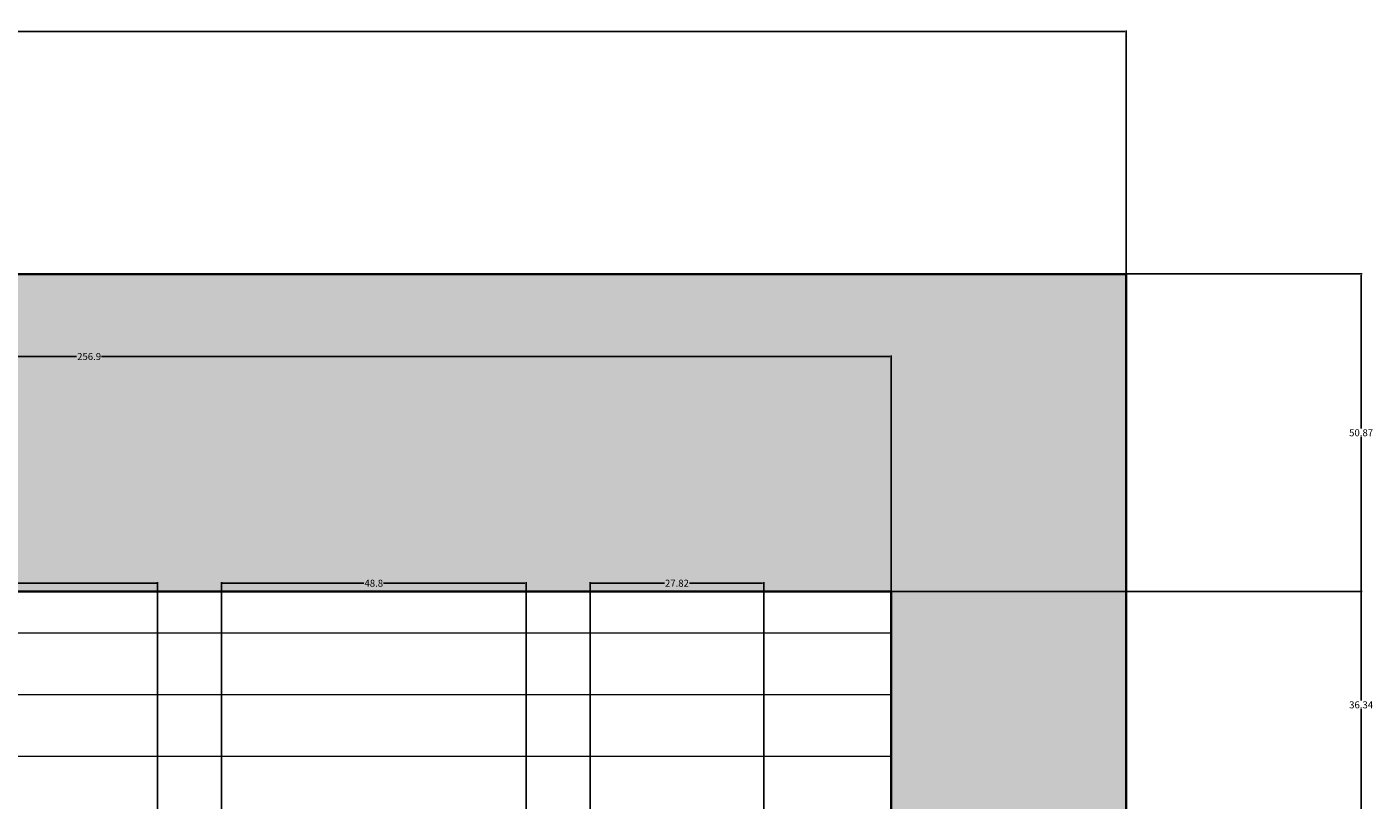
# Model space of a CAD drawing. Units: inches. Extents: x 8 to 634, y 41 to 867.
# Tile 21 of 21: x 418 to 634, y 743 to 867. Entities that reach past the tile are written whole.
import ezdxf

# ---------------------------------------------------------------- set-up
doc = ezdxf.new("R2010")
doc.units = ezdxf.units.IN
doc.header["$MEASUREMENT"] = 0
for name, color, linetype, lineweight in [('A-ANNO-DIMS', 2, 'Continuous', 18), ('A-ROOF', 7, 'Continuous', 35), ('A-ROOF-PATT', 8, 'Continuous', 9), ('A-WALL-PATT', 8, 'Continuous', 9)]:
    doc.layers.add(name, color=color, linetype=linetype, lineweight=lineweight)
doc.styles.get("Standard").update_dxf_attribs({"font": 'arial.ttf'})
doc.dimstyles.get("Standard").update_dxf_attribs({"dimtxt": 1.125, "dimasz": 0.18, "dimexe": 0.18, "dimexo": 0.0625, "dimgap": 0.09, "dimtad": 0, "dimtih": 1, "dimtoh": 1, "dimdec": 4, "dimzin": 0, "dimdsep": 46, "dimlunit": 4, "dimtxsty": 'Standard', "dimcen": 0.09, "dimadec": 0, "dimazin": 0, "dimtfac": 1, "dimtdec": 4, "dimtofl": 0, "dimtmove": 0, "dimatfit": 3, "dimfxl": 1, "dimtolj": 1, "dimtzin": 0, "dimarcsym": 0})

# ---------------------------------------------------------------- blocks, each defined once
blk = doc.blocks.new('*D19')
at = {"layer": 'A-ANNO-DIMS', "color": 0, "lineweight": -2, "transparency": 16777216}
for p, q in [((47.34, 697.73), (47.34, 866.81)), ((47.52, 866.63), (319.51, 866.63)), ((594.17, 866.63), (322.18, 866.63)), ((594.35, 827.83), (594.35, 866.81))]:
    blk.add_line(p, q, dxfattribs=at)
at = {"layer": 'A-ANNO-DIMS', "color": 0, "transparency": 16777216}
for points in [[(47.52, 866.66), (47.52, 866.6), (47.34, 866.63)], [(594.17, 866.66), (594.17, 866.6), (594.35, 866.63)]]:
    blk.add_solid(points, dxfattribs=at)
at = {"layer": 'Defpoints', "color": 0, "transparency": 16777216}
for p in [(594.35, 866.63), (594.35, 827.77), (47.34, 697.67)]:
    blk.add_point(p, dxfattribs=at)
at = {"layer": 'A-ANNO-DIMS', "color": 0, "transparency": 16777216, "insert": (320.85, 866.63), "char_height": 1.125, "attachment_point": 5}
blk.add_mtext('\\A1;547', dxfattribs=at)
blk = doc.blocks.new('*D45')
at = {"layer": 'A-ANNO-DIMS', "color": 0, "lineweight": -2, "transparency": 16777216}
for p, q in [((556.77, 776.89), (632.18, 776.89)), ((632, 776.71), (632, 759.39)), ((632, 740.74), (632, 758.06)), ((536.38, 740.56), (632.18, 740.56))]:
    blk.add_line(p, q, dxfattribs=at)
at = {"layer": 'A-ANNO-DIMS', "color": 0, "transparency": 16777216}
for points in [[(631.97, 776.71), (632.03, 776.71), (632, 776.89)], [(631.97, 740.74), (632.03, 740.74), (632, 740.56)]]:
    blk.add_solid(points, dxfattribs=at)
at = {"layer": 'Defpoints', "color": 0, "transparency": 16777216}
for p in [(556.71, 776.89), (632, 776.89), (536.32, 740.56)]:
    blk.add_point(p, dxfattribs=at)
at = {"layer": 'A-ANNO-DIMS', "color": 0, "transparency": 16777216, "insert": (632, 758.72), "char_height": 1.125, "attachment_point": 5}
blk.add_mtext('\\A1;36.34', dxfattribs=at)
blk = doc.blocks.new('*D46')
at = {"layer": 'A-ANNO-DIMS', "color": 0, "lineweight": -2, "transparency": 16777216}
for p, q in [((594.41, 827.77), (632.18, 827.77)), ((632, 827.59), (632, 802.99)), ((632, 777.07), (632, 801.67)), ((556.77, 776.89), (632.18, 776.89))]:
    blk.add_line(p, q, dxfattribs=at)
at = {"layer": 'A-ANNO-DIMS', "color": 0, "transparency": 16777216}
for points in [[(631.97, 827.59), (632.03, 827.59), (632, 827.77)], [(631.97, 777.07), (632.03, 777.07), (632, 776.89)]]:
    blk.add_solid(points, dxfattribs=at)
at = {"layer": 'Defpoints', "color": 0, "transparency": 16777216}
for p in [(594.35, 827.77), (632, 827.77), (556.71, 776.89)]:
    blk.add_point(p, dxfattribs=at)
at = {"layer": 'A-ANNO-DIMS', "color": 0, "transparency": 16777216, "insert": (632, 802.33), "char_height": 1.125, "attachment_point": 5}
blk.add_mtext('\\A1;50.87', dxfattribs=at)
blk = doc.blocks.new('*D47')
at = {"layer": 'A-ANNO-DIMS', "color": 0, "lineweight": -2, "transparency": 16777216}
for p, q in [((299.8, 776.96), (299.8, 814.72)), ((299.98, 814.54), (426.25, 814.54)), ((556.53, 814.54), (430.25, 814.54)), ((556.71, 776.96), (556.71, 814.72))]:
    blk.add_line(p, q, dxfattribs=at)
at = {"layer": 'A-ANNO-DIMS', "color": 0, "transparency": 16777216}
for points in [[(299.98, 814.57), (299.98, 814.51), (299.8, 814.54)], [(556.53, 814.57), (556.53, 814.51), (556.71, 814.54)]]:
    blk.add_solid(points, dxfattribs=at)
at = {"layer": 'Defpoints', "color": 0, "transparency": 16777216}
for p in [(556.71, 814.54), (299.8, 776.89), (556.71, 776.89)]:
    blk.add_point(p, dxfattribs=at)
at = {"layer": 'A-ANNO-DIMS', "color": 0, "transparency": 16777216, "insert": (428.25, 814.54), "char_height": 1.125, "attachment_point": 5}
blk.add_mtext('\\A1;256.9', dxfattribs=at)
blk = doc.blocks.new('*D50')
at = {"layer": 'A-ANNO-DIMS', "color": 0, "lineweight": -2, "transparency": 16777216}
for p, q in [((370.39, 740.62), (370.39, 778.39)), ((370.57, 778.21), (402.91, 778.21)), ((439.02, 778.21), (406.68, 778.21)), ((439.2, 740.62), (439.2, 778.39))]:
    blk.add_line(p, q, dxfattribs=at)
at = {"layer": 'A-ANNO-DIMS', "color": 0, "transparency": 16777216}
for points in [[(370.57, 778.24), (370.57, 778.18), (370.39, 778.21)], [(439.02, 778.24), (439.02, 778.18), (439.2, 778.21)]]:
    blk.add_solid(points, dxfattribs=at)
at = {"layer": 'Defpoints', "color": 0, "transparency": 16777216}
for p in [(439.2, 778.21), (370.39, 740.56), (439.2, 740.56)]:
    blk.add_point(p, dxfattribs=at)
at = {"layer": 'A-ANNO-DIMS', "color": 0, "transparency": 16777216, "insert": (404.79, 778.21), "char_height": 1.125, "attachment_point": 5}
blk.add_mtext('\\A1;68.81', dxfattribs=at)
blk = doc.blocks.new('*D52')
at = {"layer": 'A-ANNO-DIMS', "color": 0, "lineweight": -2, "transparency": 16777216}
for p, q in [((449.45, 740.62), (449.45, 778.39)), ((449.63, 778.21), (472.28, 778.21)), ((498.07, 778.21), (475.43, 778.21)), ((498.25, 740.62), (498.25, 778.39))]:
    blk.add_line(p, q, dxfattribs=at)
at = {"layer": 'A-ANNO-DIMS', "color": 0, "transparency": 16777216}
for points in [[(449.63, 778.24), (449.63, 778.18), (449.45, 778.21)], [(498.07, 778.24), (498.07, 778.18), (498.25, 778.21)]]:
    blk.add_solid(points, dxfattribs=at)
at = {"layer": 'Defpoints', "color": 0, "transparency": 16777216}
for p in [(498.25, 778.21), (449.45, 740.56), (498.25, 740.56)]:
    blk.add_point(p, dxfattribs=at)
at = {"layer": 'A-ANNO-DIMS', "color": 0, "transparency": 16777216, "insert": (473.85, 778.21), "char_height": 1.125, "attachment_point": 5}
blk.add_mtext('\\A1;48.8', dxfattribs=at)
blk = doc.blocks.new('*D54')
at = {"layer": 'A-ANNO-DIMS', "color": 0, "lineweight": -2, "transparency": 16777216}
for p, q in [((508.5, 740.62), (508.5, 778.39)), ((508.68, 778.21), (520.42, 778.21)), ((536.14, 778.21), (524.4, 778.21)), ((536.32, 740.62), (536.32, 778.39))]:
    blk.add_line(p, q, dxfattribs=at)
at = {"layer": 'A-ANNO-DIMS', "color": 0, "transparency": 16777216}
for points in [[(508.68, 778.24), (508.68, 778.18), (508.5, 778.21)], [(536.14, 778.24), (536.14, 778.18), (536.32, 778.21)]]:
    blk.add_solid(points, dxfattribs=at)
at = {"layer": 'Defpoints', "color": 0, "transparency": 16777216}
for p in [(536.32, 778.21), (508.5, 740.56), (536.32, 740.56)]:
    blk.add_point(p, dxfattribs=at)
at = {"layer": 'A-ANNO-DIMS', "color": 0, "transparency": 16777216, "insert": (522.41, 778.21), "char_height": 1.125, "attachment_point": 5}
blk.add_mtext('\\A1;27.82', dxfattribs=at)

msp = doc.modelspace()

# ---------------------------------------------------------------- hatches: boundary and pattern name
at = {"layer": 'A-ROOF-PATT', "transparency": 33554687}
h = msp.add_hatch(dxfattribs=at)
h.set_pattern_fill('AR-CONC', color=256, scale=2.2, angle=135)
h.paths.add_polyline_path([(262.2266, 828.9821), (144.3564, 828.9821), (144.3564, 697.6655), (262.2266, 785.231), (245.114, 785.231), (245.114, 792.8938), (262.2266, 792.8938)])
h.paths.add_polyline_path([(594.3501, 827.7671), (262.2266, 827.7671), (262.2266, 792.8938), (262.2266, 697.6655), (299.7961, 697.6655), (299.7961, 776.8929), (556.7072, 776.8929), (556.7072, 774.3342), (556.7072, 697.6655), (594.3501, 697.6655)])
at = {"layer": 'A-WALL-PATT', "transparency": 33554687}
h = msp.add_hatch(dxfattribs=at)
h.set_pattern_fill('ANSI31', color=256, scale=79, angle=135)
h.paths.add_polyline_path([(539.0002, 276.166), (499.4677, 276.166), (418.2881, 276.166), (418.2881, 228.4951), (435.5682, 228.4951), (539.0002, 228.4951)])
h.paths.add_polyline_path([(539.0002, 228.4951), (435.5682, 228.4951), (418.2881, 228.4951), (418.2881, 112.2342), (439.3242, 112.2342), (539.0002, 112.2342)])
h.paths.add_polyline_path([(518.1129, 124.2342), (473.3277, 124.2342), (473.3277, 216.4951), (518.1129, 216.4951)], flags=16)
h.paths.add_polyline_path([(451.2116, 124.2342), (427.4368, 124.2342), (427.4368, 216.4951), (451.2116, 216.4951)], flags=16)
h.paths.add_polyline_path([(539.0002, 112.2342), (439.3242, 112.2342), (418.2881, 112.2342), (418.2881, 91.5417), (539.0002, 91.5417)])
h.paths.add_polyline_path([(539.0002, 392.4268), (427.4368, 392.4268), (418.2881, 392.4268), (418.2881, 391.7598), (418.2881, 276.166), (499.4677, 276.166), (539.0002, 276.166)])
h.paths.add_polyline_path([(518.1129, 288.166), (473.3277, 288.166), (473.3277, 380.4268), (518.1129, 380.4268)], flags=16)
h.paths.add_polyline_path([(451.2116, 288.166), (427.4368, 288.166), (427.4368, 380.4268), (451.2116, 380.4268)], flags=16)
h.paths.add_polyline_path([(539.0002, 451.6305), (427.4368, 452.9097), (418.2881, 452.9097), (418.2881, 392.4268), (427.4368, 392.4268), (539.0002, 392.4268)])
h.paths.add_polyline_path([(539.0002, 569.1705), (427.4368, 569.1705), (418.2881, 569.1705), (418.2881, 452.9097), (427.4368, 452.9097), (539.0002, 451.6305)])
h.paths.add_polyline_path([(473.3277, 557.1705), (518.1129, 557.1705), (518.1129, 464.9097), (473.3277, 464.9097)], flags=16)
h.paths.add_polyline_path([(451.2116, 557.1705), (451.2116, 464.9097), (427.4368, 464.9097), (427.4368, 557.1705)], flags=16)
h.paths.add_polyline_path([(539.0002, 619.6298), (418.2881, 619.6298), (418.2881, 569.1705), (427.4368, 569.1705), (539.0002, 569.1705)])
h.paths.add_polyline_path([(556.7072, 774.3342), (556.7072, 776.8929), (299.7961, 776.8929), (299.7961, 697.6655), (322.56, 697.6655), (322.56, 740.5561), (355.7466, 740.5561), (355.7466, 697.6655), (360.785, 697.6655), (370.3877, 697.6655), (370.3877, 740.5561), (439.201, 740.5561), (439.201, 691.978), (449.4498, 691.978), (449.4498, 740.5561), (498.2535, 740.5561), (498.2535, 691.978), (508.5023, 691.978), (508.5023, 740.5561), (536.3204, 740.5561), (536.3204, 691.978), (539.0002, 691.978), (539.0002, 697.6655), (556.7072, 697.6655)])

# ---------------------------------------------------------------- linework, layer by layer
at = {"layer": 'A-ROOF'}
for p, q in [((594.3501, 827.7671), (262.2266, 827.7671)), ((594.3501, 697.6655), (594.3501, 827.7671)), ((299.7961, 776.8929), (556.7072, 776.8929)), ((556.7072, 774.3342), (556.7072, 776.8929)), ((556.7072, 774.3342), (556.7072, 697.6655))]:
    msp.add_line(p, q, dxfattribs=at)

# ---------------------------------------------------------------- dimensions: what is measured, and where the dimension line sits
at = {"layer": 'A-ANNO-DIMS'}
for base, p1, p2, override, picture, middle in [((594.3501, 866.6321), (47.3401, 697.6655), (594.3501, 827.7671), {"dimdec": 0, "dimlfac": 1, "dimrnd": 0, "dimzin": 0, "dimdsep": 46, "dimlunit": 2}, '*D19', (320.8451, 866.6321)), ((556.7072, 814.5429), (299.7961, 776.8929), (556.7072, 776.8929), {"dimdec": 1, "dimlfac": 1, "dimrnd": 0, "dimzin": 0, "dimdsep": 46, "dimlunit": 2}, '*D47', (428.2516, 814.5429)), ((439.201, 778.2061), (370.3877, 740.5561), (439.201, 740.5561), {"dimdec": 2, "dimlfac": 1, "dimrnd": 0, "dimzin": 0, "dimdsep": 46, "dimlunit": 2}, '*D50', (404.7943, 778.2061)), ((498.2535, 778.2061), (449.4498, 740.5561), (498.2535, 740.5561), {"dimdec": 1, "dimlfac": 1, "dimrnd": 0, "dimzin": 0, "dimdsep": 46, "dimlunit": 2}, '*D52', (473.8516, 778.2061)), ((536.3204, 778.2061), (508.5023, 740.5561), (536.3204, 740.5561), {"dimdec": 2, "dimlfac": 1, "dimrnd": 0, "dimzin": 0, "dimdsep": 46, "dimlunit": 2}, '*D54', (522.4114, 778.2061))]:
    dim = msp.add_linear_dim(base=base, p1=p1, p2=p2, dimstyle='Standard', override=override, dxfattribs=at)
    dim.commit()
    dim.dimension.update_dxf_attribs({"geometry": picture, "text_midpoint": middle})
for base, p1, p2, picture, middle in [((632.0001, 827.7671), (556.7072, 776.8929), (594.3501, 827.7671), '*D46', (632.0001, 802.33)), ((632.0001, 776.8929), (536.3204, 740.5561), (556.7072, 776.8929), '*D45', (632.0001, 758.7245))]:
    dim = msp.add_linear_dim(base=base, p1=p1, p2=p2, angle=90, dimstyle='Standard', override={"dimdec": 2, "dimlfac": 1, "dimrnd": 0, "dimzin": 0, "dimdsep": 46, "dimlunit": 2}, dxfattribs=at)
    dim.commit()
    dim.dimension.update_dxf_attribs({"geometry": picture, "text_midpoint": middle})

doc.saveas('drawing.dxf')
